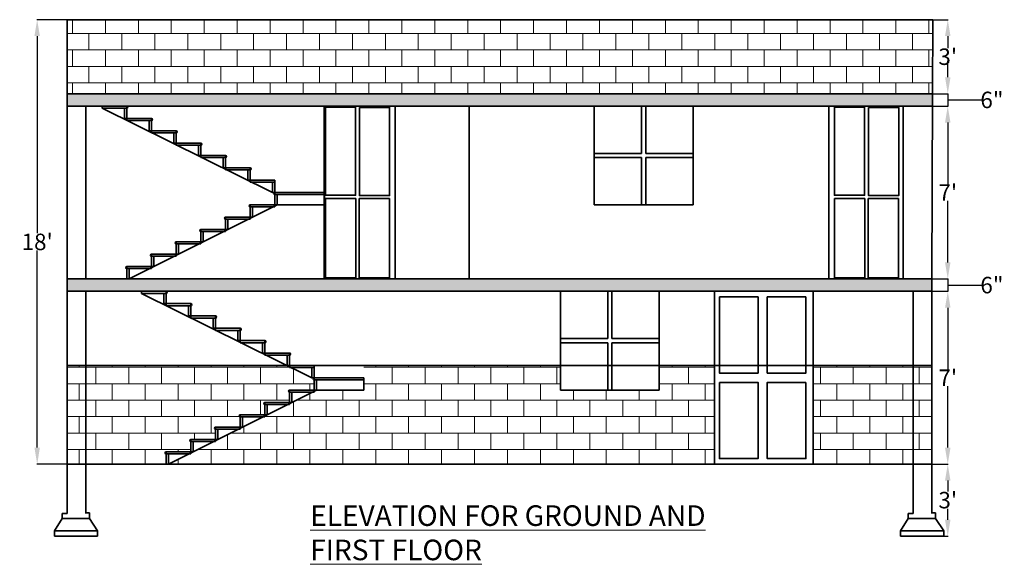
# Model space of a CAD drawing. Units: inches. Extents: x 179 to 2009, y 628 to 2084.
# Tile 5 of 5: x 1531 to 2009, y 888 to 1153. Entities that reach past the tile are written whole.
import ezdxf

# ---------------------------------------------------------------- set-up
doc = ezdxf.new("R2010")
doc.units = ezdxf.units.IN
doc.header["$MEASUREMENT"] = 0
for name, color, linetype, lineweight in [('A-ANNO-DIMS', 2, 'Continuous', 18), ('A-ANNO-TEXT', 7, 'Continuous', 18), ('A-ELEV', 7, 'Continuous', 35), ('A-ELEV-PATT', 8, 'Continuous', 13)]:
    doc.layers.add(name, color=color, linetype=linetype, lineweight=lineweight)
doc.styles.get("Standard").update_dxf_attribs({"font": 'arial.ttf'})
doc.dimstyles.get("Standard").update_dxf_attribs({"dimtxt": 8, "dimasz": 8, "dimexe": 0.18, "dimexo": 0.0625, "dimgap": 0.09, "dimtad": 0, "dimtih": 1, "dimtoh": 1, "dimdec": 0, "dimzin": 0, "dimdsep": 46, "dimlunit": 3, "dimtxsty": 'Standard', "dimcen": 0.09, "dimadec": 0, "dimazin": 0, "dimtfac": 1, "dimtdec": 0, "dimtofl": 0, "dimtmove": 0, "dimatfit": 3, "dimfxl": 1, "dimtolj": 1, "dimtzin": 0, "dimarcsym": 0})
pattern_1 = [(50, (0, 0), (7.172602, -0.627521), [0.75, -8.25]), (355, (0, 0), (-1.387513, 7.521921), [0.6, -6.6]), (100.45144, (0.598, -0.052), (5.785088, 6.8944), [0.637402, -7.01142]), (46.1842, (0, 2), (10.672413, -1.655193), [1.125, -12.375]), (96.63564, (0.889, 1.862), (9.34662, 9.741186), [0.956103, -10.51714]), (351.18416, (0, 2), (9.34662, 9.741186), [0.9, -9.9]), (21, (1, 1.5), (5.96907, -4.026189), [0.75, -8.25]), (326, (1, 1.5), (2.433153, 7.2515), [0.6, -6.6]), (71.45144, (1.4974, 1.1645), (8.402224, 3.225312), [0.637402, -7.01142]), (37.5, (0, 0), (0.1215986, 3.3289385), [0, -6.52, 0, -6.7, 0, -6.625]), (7.5, (0, 0), (2.6306954, 3.944117), [0, -3.82, 0, -6.37, 0, -2.525]), (327.5, (-2.23, 0), (5.3382244, -0.2255487), [0, -2.5, 0, -7.8, 0, -10.35]), (317.5, (-3.23, 0), (5.831862, 1.00105), [0, -3.25, 0, -5.18, 0, -7.35])]

# ---------------------------------------------------------------- blocks, each defined once
blk = doc.blocks.new('*D24')
at = {"layer": 'A-ANNO-DIMS', "color": 0, "lineweight": -2, "transparency": 16777216}
for p, q in [((1554.1, 1152.94), (1539.38, 1152.94)), ((1539.56, 1144.94), (1539.56, 1049.11)), ((1539.56, 944.94), (1539.56, 1040.76)), ((1554.1, 936.94), (1539.38, 936.94))]:
    blk.add_line(p, q, dxfattribs=at)
at = {"layer": 'A-ANNO-DIMS', "color": 0, "transparency": 16777216}
for points in [[(1538.22, 1144.94), (1540.89, 1144.94), (1539.56, 1152.94)], [(1538.22, 944.94), (1540.89, 944.94), (1539.56, 936.94)]]:
    blk.add_solid(points, dxfattribs=at)
at = {"layer": 'Defpoints', "color": 0, "transparency": 16777216}
for p in [(1554.16, 1152.94), (1539.56, 936.94), (1554.16, 936.94)]:
    blk.add_point(p, dxfattribs=at)
at = {"layer": 'A-ANNO-DIMS', "color": 0, "transparency": 16777216, "insert": (1539.56, 1044.94), "char_height": 8, "attachment_point": 5}
blk.add_mtext("\\A1;18'", dxfattribs=at)
blk = doc.blocks.new('*D25')
at = {"layer": 'A-ANNO-DIMS', "color": 0, "lineweight": -2, "transparency": 16777216}
for p, q in [((1974.69, 1152.94), (1982.07, 1152.94)), ((1981.89, 1144.94), (1981.89, 1139.11)), ((1981.89, 1124.94), (1981.89, 1130.76)), ((1974.69, 1116.94), (1982.07, 1116.94))]:
    blk.add_line(p, q, dxfattribs=at)
at = {"layer": 'A-ANNO-DIMS', "color": 0, "transparency": 16777216}
for points in [[(1980.56, 1144.94), (1983.22, 1144.94), (1981.89, 1152.94)], [(1980.56, 1124.94), (1983.22, 1124.94), (1981.89, 1116.94)]]:
    blk.add_solid(points, dxfattribs=at)
at = {"layer": 'Defpoints', "color": 0, "transparency": 16777216}
for p in [(1974.62, 1152.94), (1974.62, 1116.94), (1981.89, 1116.94)]:
    blk.add_point(p, dxfattribs=at)
at = {"layer": 'A-ANNO-DIMS', "color": 0, "transparency": 16777216, "insert": (1981.89, 1134.94), "char_height": 8, "attachment_point": 5}
blk.add_mtext("\\A1;3'", dxfattribs=at)
blk = doc.blocks.new('*D26')
at = {"layer": 'A-ANNO-DIMS', "color": 0, "lineweight": -2, "transparency": 16777216}
for p, q in [((1981.89, 1124.94), (1981.89, 1132.94)), ((1974.69, 1116.94), (1982.07, 1116.94)), ((1981.89, 1116.94), (1981.89, 1110.94)), ((1974.53, 1110.94), (1982.07, 1110.94)), ((1981.89, 1113.94), (1998.45, 1113.94)), ((1998.45, 1113.94), (1998.63, 1113.94)), ((1981.89, 1102.94), (1981.89, 1094.94))]:
    blk.add_line(p, q, dxfattribs=at)
at = {"layer": 'A-ANNO-DIMS', "color": 0, "transparency": 16777216}
for points in [[(1980.56, 1124.94), (1983.22, 1124.94), (1981.89, 1116.94)], [(1980.56, 1102.94), (1983.22, 1102.94), (1981.89, 1110.94)]]:
    blk.add_solid(points, dxfattribs=at)
at = {"layer": 'Defpoints', "color": 0, "transparency": 16777216}
for p in [(1974.62, 1116.94), (1974.47, 1110.94), (1981.89, 1110.94)]:
    blk.add_point(p, dxfattribs=at)
at = {"layer": 'A-ANNO-DIMS', "color": 0, "transparency": 16777216, "insert": (2003.34, 1113.94), "char_height": 8, "attachment_point": 5}
blk.add_mtext('\\A1;6"', dxfattribs=at)
blk = doc.blocks.new('*D27')
at = {"layer": 'A-ANNO-DIMS', "color": 0, "lineweight": -2, "transparency": 16777216}
for p, q in [((1974.53, 1110.94), (1982.07, 1110.94)), ((1981.89, 1102.94), (1981.89, 1073.03)), ((1981.89, 1034.94), (1981.89, 1064.85)), ((1974.22, 1026.94), (1982.07, 1026.94))]:
    blk.add_line(p, q, dxfattribs=at)
at = {"layer": 'A-ANNO-DIMS', "color": 0, "transparency": 16777216}
for points in [[(1980.56, 1102.94), (1983.22, 1102.94), (1981.89, 1110.94)], [(1980.56, 1034.94), (1983.22, 1034.94), (1981.89, 1026.94)]]:
    blk.add_solid(points, dxfattribs=at)
at = {"layer": 'Defpoints', "color": 0, "transparency": 16777216}
for p in [(1974.47, 1110.94), (1974.16, 1026.94), (1981.89, 1026.94)]:
    blk.add_point(p, dxfattribs=at)
at = {"layer": 'A-ANNO-DIMS', "color": 0, "transparency": 16777216, "insert": (1981.89, 1068.94), "char_height": 8, "attachment_point": 5}
blk.add_mtext("\\A1;7'", dxfattribs=at)
blk = doc.blocks.new('*D28')
at = {"layer": 'A-ANNO-DIMS', "color": 0, "lineweight": -2, "transparency": 16777216}
for p, q in [((1981.89, 1034.94), (1981.89, 1042.94)), ((1974.22, 1026.94), (1982.07, 1026.94)), ((1981.89, 1026.94), (1981.89, 1020.94)), ((1981.89, 1023.94), (1998.45, 1023.94)), ((1998.45, 1023.94), (1998.63, 1023.94)), ((1974.22, 1020.94), (1982.07, 1020.94)), ((1981.89, 1012.94), (1981.89, 1004.94))]:
    blk.add_line(p, q, dxfattribs=at)
at = {"layer": 'A-ANNO-DIMS', "color": 0, "transparency": 16777216}
for points in [[(1980.56, 1034.94), (1983.22, 1034.94), (1981.89, 1026.94)], [(1980.56, 1012.94), (1983.22, 1012.94), (1981.89, 1020.94)]]:
    blk.add_solid(points, dxfattribs=at)
at = {"layer": 'Defpoints', "color": 0, "transparency": 16777216}
for p in [(1974.16, 1026.94), (1974.16, 1020.94), (1981.89, 1020.94)]:
    blk.add_point(p, dxfattribs=at)
at = {"layer": 'A-ANNO-DIMS', "color": 0, "transparency": 16777216, "insert": (2003.34, 1023.94), "char_height": 8, "attachment_point": 5}
blk.add_mtext('\\A1;6"', dxfattribs=at)
blk = doc.blocks.new('*D29')
at = {"layer": 'A-ANNO-DIMS', "color": 0, "lineweight": -2, "transparency": 16777216}
for p, q in [((1974.22, 1020.94), (1982.07, 1020.94)), ((1981.89, 1012.94), (1981.89, 983.03)), ((1981.89, 944.94), (1981.89, 974.85)), ((1974.22, 936.94), (1982.07, 936.94))]:
    blk.add_line(p, q, dxfattribs=at)
at = {"layer": 'A-ANNO-DIMS', "color": 0, "transparency": 16777216}
for points in [[(1980.56, 1012.94), (1983.22, 1012.94), (1981.89, 1020.94)], [(1980.56, 944.94), (1983.22, 944.94), (1981.89, 936.94)]]:
    blk.add_solid(points, dxfattribs=at)
at = {"layer": 'Defpoints', "color": 0, "transparency": 16777216}
for p in [(1974.16, 1020.94), (1974.16, 936.94), (1981.89, 936.94)]:
    blk.add_point(p, dxfattribs=at)
at = {"layer": 'A-ANNO-DIMS', "color": 0, "transparency": 16777216, "insert": (1981.89, 978.94), "char_height": 8, "attachment_point": 5}
blk.add_mtext("\\A1;7'", dxfattribs=at)
blk = doc.blocks.new('*D30')
at = {"layer": 'A-ANNO-DIMS', "color": 0, "lineweight": -2, "transparency": 16777216}
for p, q in [((1974.22, 936.94), (1982.07, 936.94)), ((1981.89, 928.94), (1981.89, 923.61)), ((1981.89, 909.94), (1981.89, 915.26)), ((1977.81, 901.94), (1982.07, 901.94))]:
    blk.add_line(p, q, dxfattribs=at)
at = {"layer": 'A-ANNO-DIMS', "color": 0, "transparency": 16777216}
for points in [[(1980.56, 928.94), (1983.22, 928.94), (1981.89, 936.94)], [(1980.56, 909.94), (1983.22, 909.94), (1981.89, 901.94)]]:
    blk.add_solid(points, dxfattribs=at)
at = {"layer": 'Defpoints', "color": 0, "transparency": 16777216}
for p in [(1974.16, 936.94), (1977.75, 901.94), (1981.89, 901.94)]:
    blk.add_point(p, dxfattribs=at)
at = {"layer": 'A-ANNO-DIMS', "color": 0, "transparency": 16777216, "insert": (1981.89, 919.44), "char_height": 8, "attachment_point": 5}
blk.add_mtext("\\A1;3'", dxfattribs=at)

msp = doc.modelspace()

# ---------------------------------------------------------------- hatches: boundary and pattern name
at = {"layer": 'A-ELEV-PATT'}
h = msp.add_hatch(dxfattribs=at)
h.set_pattern_fill('AR-B816', color=256)
h.set_pattern_definition([(0, (500.695, 474.206), (0, 8), []), (90, (500.695, 474.206), (-8, 8), [8, -8])])
h.paths.add_polyline_path([(1974.49, 1116.94), (1974.62, 1152.94), (1554.16, 1152.94), (1554.16, 1116.94)])
h = msp.add_hatch(dxfattribs=at)
h.set_pattern_fill('AR-CONC', color=256)
h.set_pattern_definition(pattern_1)
h.paths.add_polyline_path([(1974.49, 1116.94), (1554.16, 1116.94), (1554.16, 1110.94), (1974.47, 1110.94)])
h = msp.add_hatch(dxfattribs=at)
h.set_pattern_fill('AR-CONC', color=256)
h.set_pattern_definition(pattern_1)
h.paths.add_polyline_path([(1974.16, 1026.94), (1554.16, 1026.94), (1554.16, 1020.94), (1974.16, 1020.94)])
h = msp.add_hatch(dxfattribs=at)
h.set_pattern_fill('AR-B816', color=256)
h.paths.add_polyline_path([(1650.16, 965.94, -1), (1650.16, 966.94), (1662.16, 966.94), (1662.16, 971.94, -1), (1662.16, 972.94), (1674.16, 972.94), (1674.16, 977.94, -1), (1674.16, 978.94), (1673.02, 978.94), (1662.92, 983.94), (1662.16, 983.94), (1662.16, 984.31), (1660.9, 984.94), (1563.16, 984.94), (1563.16, 936.94), (1602.16, 936.94), (1602.16, 941.94, -1), (1602.16, 942.94), (1614.16, 942.94), (1614.16, 947.94, -1), (1614.16, 948.94), (1626.16, 948.94), (1626.16, 953.94, -1), (1626.16, 954.94), (1638.16, 954.94), (1638.16, 959.94, -1), (1638.16, 960.94), (1650.16, 960.94)])
h.paths.add_polyline_path([(1698.16, 972.94), (1675.3, 972.94), (1674.16, 972.37), (1674.16, 971.94), (1673.3, 971.94), (1662.16, 966.37), (1662.16, 965.94), (1661.3, 965.94), (1650.16, 960.37), (1650.16, 959.94), (1649.3, 959.94), (1638.16, 954.37), (1638.16, 953.94), (1637.3, 953.94), (1626.16, 948.37), (1626.16, 947.94), (1625.3, 947.94), (1614.16, 942.37), (1614.16, 941.94), (1613.3, 941.94), (1603.3, 936.94), (1698.16, 936.94)])
h.paths.add_polyline_path([(1563.16, 984.94), (1554.16, 984.94), (1554.16, 936.94), (1563.16, 936.94)])
h.paths.add_polyline_path([(1868.5, 984.94), (1841.75, 984.94), (1841.75, 972.94), (1793.75, 972.94), (1793.75, 984.94), (1698.16, 984.94), (1698.16, 936.94), (1868.5, 936.94)])
h.paths.add_polyline_path([(1965.16, 984.94), (1916.5, 984.94), (1916.5, 936.94), (1965.16, 936.94)])
h.paths.add_polyline_path([(1974.16, 984.94), (1965.16, 984.94), (1965.16, 936.94), (1974.16, 936.94)])

# ---------------------------------------------------------------- linework, layer by layer
at = {"layer": 'A-ELEV'}
for p, q in [((1554.16, 1116.94), (1554.16, 1152.94)), ((1554.16, 1152.94), (1974.62, 1152.94)), ((1974.62, 1152.94), (1974.49, 1116.94)), ((1554.16, 1116.94), (1974.49, 1116.94)), ((1554.16, 1116.94), (1554.16, 1026.94)), ((1974.49, 1116.94), (1974.16, 1026.94)), ((1554.16, 1110.94), (1974.47, 1110.94)), ((1563.16, 1026.94), (1563.16, 1110.94)), ((1583.07, 1110.94), (1571.07, 1110.94)), ((1571.07, 1110.94), (1571.07, 1109.94)), ((1571.07, 1109.94), (1583.07, 1109.94)), ((1571.07, 1109.94), (1653.94, 1068.94)), ((1581.94, 1109.94), (1581.94, 1104.94)), ((1583.07, 1104.94), (1583.07, 1110.94)), ((1678.94, 1026.94), (1678.94, 1110.94)), ((1713.45, 1026.94), (1713.45, 1110.94)), ((1749.45, 1026.94), (1749.45, 1110.94)), ((1810.16, 1062.94), (1810.16, 1110.94)), ((1833.16, 1087.94), (1833.16, 1110.94)), ((1835.16, 1087.94), (1835.16, 1110.94)), ((1858.16, 1062.94), (1858.16, 1110.94)), ((1924.18, 1026.94), (1924.18, 1110.94)), ((1960.18, 1026.94), (1960.18, 1110.94)), ((1583.07, 1104.94), (1581.94, 1104.94)), ((1595.07, 1104.94), (1583.07, 1104.94)), ((1583.07, 1104.94), (1583.07, 1103.94)), ((1595.07, 1098.94), (1595.07, 1104.94)), ((1583.07, 1103.94), (1595.07, 1103.94)), ((1593.94, 1103.94), (1593.94, 1098.94)), ((1595.07, 1098.94), (1593.94, 1098.94)), ((1607.07, 1098.94), (1595.07, 1098.94)), ((1595.07, 1098.94), (1595.07, 1097.94)), ((1595.07, 1097.94), (1607.07, 1097.94)), ((1605.94, 1097.94), (1605.94, 1092.94)), ((1607.07, 1092.94), (1607.07, 1098.94)), ((1607.07, 1092.94), (1605.94, 1092.94)), ((1619.07, 1092.94), (1607.07, 1092.94)), ((1607.07, 1092.94), (1607.07, 1091.94)), ((1607.07, 1091.94), (1619.07, 1091.94)), ((1617.94, 1091.94), (1617.94, 1086.94)), ((1619.07, 1086.94), (1619.07, 1092.94)), ((1619.07, 1086.94), (1617.94, 1086.94)), ((1631.07, 1086.94), (1619.07, 1086.94)), ((1619.07, 1086.94), (1619.07, 1085.94)), ((1619.07, 1085.94), (1631.07, 1085.94)), ((1629.94, 1085.94), (1629.94, 1080.94)), ((1631.07, 1080.94), (1631.07, 1086.94)), ((1833.16, 1087.94), (1810.16, 1087.94)), ((1833.16, 1085.94), (1810.16, 1085.94)), ((1833.16, 1062.94), (1833.16, 1085.94)), ((1858.16, 1087.94), (1835.16, 1087.94)), ((1835.16, 1062.94), (1835.16, 1085.94)), ((1858.16, 1085.94), (1835.16, 1085.94)), ((1631.07, 1080.94), (1629.94, 1080.94)), ((1643.07, 1080.94), (1631.07, 1080.94)), ((1631.07, 1080.94), (1631.07, 1079.94)), ((1631.07, 1079.94), (1643.07, 1079.94)), ((1641.94, 1079.94), (1641.94, 1074.94)), ((1643.07, 1074.94), (1643.07, 1080.94)), ((1643.07, 1074.94), (1641.94, 1074.94)), ((1655.07, 1074.94), (1643.07, 1074.94)), ((1643.07, 1074.94), (1643.07, 1073.94)), ((1643.07, 1073.94), (1655.07, 1073.94)), ((1653.94, 1073.94), (1653.94, 1068.94)), ((1655.07, 1068.94), (1655.07, 1074.94)), ((1655.07, 1068.94), (1653.94, 1068.94)), ((1655.07, 1062.94), (1655.07, 1068.94)), ((1655.07, 1068.94), (1667.07, 1068.94)), ((1667.07, 1067.94), (1655.07, 1067.94)), ((1656.21, 1067.94), (1656.21, 1062.94)), ((1667.07, 1068.94), (1679.07, 1068.94)), ((1667.07, 1067.94), (1679.07, 1067.94)), ((1679.07, 1068.94), (1679.07, 1062.94)), ((1584.21, 1026.94), (1656.21, 1062.94)), ((1643.07, 1056.94), (1643.07, 1062.94)), ((1643.07, 1062.94), (1655.07, 1062.94)), ((1655.07, 1061.94), (1643.07, 1061.94)), ((1644.21, 1061.94), (1644.21, 1056.94)), ((1655.07, 1062.94), (1655.07, 1061.94)), ((1655.07, 1062.94), (1656.21, 1062.94)), ((1656.21, 1062.94), (1679.07, 1062.94)), ((1810.16, 1062.94), (1858.16, 1062.94)), ((1631.07, 1050.94), (1631.07, 1056.94)), ((1631.07, 1056.94), (1643.07, 1056.94)), ((1643.07, 1055.94), (1631.07, 1055.94)), ((1632.21, 1055.94), (1632.21, 1050.94)), ((1643.07, 1056.94), (1643.07, 1055.94)), ((1643.07, 1056.94), (1644.21, 1056.94)), ((1619.07, 1044.94), (1619.07, 1050.94)), ((1619.07, 1050.94), (1631.07, 1050.94)), ((1631.07, 1049.94), (1619.07, 1049.94)), ((1620.21, 1049.94), (1620.21, 1044.94)), ((1631.07, 1050.94), (1631.07, 1049.94)), ((1631.07, 1050.94), (1632.21, 1050.94)), ((1607.07, 1038.94), (1607.07, 1044.94)), ((1607.07, 1044.94), (1619.07, 1044.94)), ((1619.07, 1043.94), (1607.07, 1043.94)), ((1608.21, 1043.94), (1608.21, 1038.94)), ((1619.07, 1044.94), (1619.07, 1043.94)), ((1619.07, 1044.94), (1620.21, 1044.94)), ((1595.07, 1032.94), (1595.07, 1038.94)), ((1595.07, 1038.94), (1607.07, 1038.94)), ((1607.07, 1037.94), (1595.07, 1037.94)), ((1596.21, 1037.94), (1596.21, 1032.94)), ((1607.07, 1038.94), (1607.07, 1037.94)), ((1607.07, 1038.94), (1608.21, 1038.94)), ((1583.07, 1026.94), (1583.07, 1032.94)), ((1583.07, 1032.94), (1595.07, 1032.94)), ((1595.07, 1031.94), (1583.07, 1031.94)), ((1584.21, 1031.94), (1584.21, 1026.94)), ((1595.07, 1032.94), (1595.07, 1031.94)), ((1595.07, 1032.94), (1596.21, 1032.94)), ((1554.16, 1026.94), (1974.16, 1026.94)), ((1554.16, 1026.94), (1554.16, 936.94)), ((1554.16, 1026.94), (1974.16, 1026.94)), ((1583.07, 1026.94), (1584.21, 1026.94)), ((1974.16, 1026.94), (1974.16, 936.94)), ((1554.16, 1020.94), (1974.16, 1020.94)), ((1563.16, 936.94), (1563.16, 1020.94)), ((1602.16, 1020.94), (1590.16, 1020.94)), ((1590.16, 1020.94), (1590.16, 1019.94)), ((1590.16, 1019.94), (1602.16, 1019.94)), ((1590.16, 1019.94), (1673.02, 978.94)), ((1601.02, 1019.94), (1601.02, 1014.94)), ((1602.16, 1014.94), (1602.16, 1020.94)), ((1793.75, 972.94), (1793.75, 1020.94)), ((1816.75, 997.94), (1816.75, 1020.94)), ((1818.75, 997.94), (1818.75, 1020.94)), ((1841.75, 972.94), (1841.75, 1020.94)), ((1868.5, 936.94), (1868.5, 1020.94)), ((1916.5, 936.94), (1916.5, 1020.94)), ((1965.16, 936.94), (1965.16, 1020.94)), ((1602.16, 1014.94), (1601.02, 1014.94)), ((1614.16, 1014.94), (1602.16, 1014.94)), ((1602.16, 1014.94), (1602.16, 1013.94)), ((1614.16, 1008.94), (1614.16, 1014.94)), ((1602.16, 1013.94), (1614.16, 1013.94)), ((1613.02, 1013.94), (1613.02, 1008.94)), ((1614.16, 1008.94), (1613.02, 1008.94)), ((1626.16, 1008.94), (1614.16, 1008.94)), ((1614.16, 1008.94), (1614.16, 1007.94)), ((1614.16, 1007.94), (1626.16, 1007.94)), ((1625.02, 1007.94), (1625.02, 1002.94)), ((1626.16, 1002.94), (1626.16, 1008.94)), ((1626.16, 1002.94), (1625.02, 1002.94)), ((1638.16, 1002.94), (1626.16, 1002.94)), ((1626.16, 1002.94), (1626.16, 1001.94)), ((1626.16, 1001.94), (1638.16, 1001.94)), ((1637.02, 1001.94), (1637.02, 996.94)), ((1638.16, 996.94), (1638.16, 1002.94)), ((1638.16, 996.94), (1637.02, 996.94)), ((1650.16, 996.94), (1638.16, 996.94)), ((1638.16, 996.94), (1638.16, 995.94)), ((1638.16, 995.94), (1650.16, 995.94)), ((1649.02, 995.94), (1649.02, 990.94)), ((1650.16, 990.94), (1650.16, 996.94)), ((1816.75, 997.94), (1793.75, 997.94)), ((1816.75, 995.94), (1793.75, 995.94)), ((1816.75, 972.94), (1816.75, 995.94)), ((1841.75, 997.94), (1818.75, 997.94)), ((1818.75, 972.94), (1818.75, 995.94)), ((1841.75, 995.94), (1818.75, 995.94)), ((1650.16, 990.94), (1649.02, 990.94)), ((1662.16, 990.94), (1650.16, 990.94)), ((1650.16, 990.94), (1650.16, 989.94)), ((1662.16, 984.94), (1662.16, 990.94)), ((1650.16, 989.94), (1662.16, 989.94)), ((1661.02, 989.94), (1661.02, 984.94)), ((1554.16, 984.94), (1974.16, 984.94)), ((1662.16, 984.94), (1661.02, 984.94)), ((1674.16, 984.94), (1662.16, 984.94)), ((1662.16, 984.94), (1662.16, 983.94)), ((1662.16, 983.94), (1674.16, 983.94)), ((1673.02, 983.94), (1673.02, 978.94)), ((1674.16, 978.94), (1674.16, 984.94)), ((1674.16, 978.94), (1673.02, 978.94)), ((1674.16, 972.94), (1674.16, 978.94)), ((1674.16, 978.94), (1686.16, 978.94)), ((1686.16, 977.94), (1674.16, 977.94)), ((1675.3, 977.94), (1675.3, 972.94)), ((1686.16, 978.94), (1698.16, 978.94)), ((1686.16, 977.94), (1698.16, 977.94)), ((1698.16, 978.94), (1698.16, 972.94)), ((1603.3, 936.94), (1675.3, 972.94)), ((1662.16, 966.94), (1662.16, 972.94)), ((1662.16, 972.94), (1674.16, 972.94)), ((1674.16, 971.94), (1662.16, 971.94)), ((1663.3, 971.94), (1663.3, 966.94)), ((1674.16, 972.94), (1674.16, 971.94)), ((1674.16, 972.94), (1675.3, 972.94)), ((1675.3, 972.94), (1698.16, 972.94)), ((1793.75, 972.94), (1841.75, 972.94)), ((1650.16, 960.94), (1650.16, 966.94)), ((1650.16, 966.94), (1662.16, 966.94)), ((1662.16, 966.94), (1662.16, 965.94)), ((1662.16, 966.94), (1663.3, 966.94)), ((1662.16, 965.94), (1650.16, 965.94)), ((1651.3, 965.94), (1651.3, 960.94)), ((1638.16, 954.94), (1638.16, 960.94)), ((1638.16, 960.94), (1650.16, 960.94)), ((1650.16, 959.94), (1638.16, 959.94)), ((1639.3, 959.94), (1639.3, 954.94)), ((1650.16, 960.94), (1650.16, 959.94)), ((1650.16, 960.94), (1651.3, 960.94)), ((1626.16, 948.94), (1626.16, 954.94)), ((1626.16, 954.94), (1638.16, 954.94)), ((1638.16, 953.94), (1626.16, 953.94)), ((1627.3, 953.94), (1627.3, 948.94)), ((1638.16, 954.94), (1638.16, 953.94)), ((1638.16, 954.94), (1639.3, 954.94)), ((1614.16, 942.94), (1614.16, 948.94)), ((1614.16, 948.94), (1626.16, 948.94)), ((1626.16, 947.94), (1614.16, 947.94)), ((1615.3, 947.94), (1615.3, 942.94)), ((1626.16, 948.94), (1626.16, 947.94)), ((1626.16, 948.94), (1627.3, 948.94)), ((1602.16, 936.94), (1602.16, 942.94)), ((1602.16, 942.94), (1614.16, 942.94)), ((1614.16, 942.94), (1614.16, 941.94)), ((1614.16, 942.94), (1615.3, 942.94)), ((1614.16, 941.94), (1602.16, 941.94)), ((1603.3, 941.94), (1603.3, 936.94)), ((1554.16, 936.94), (1974.16, 936.94)), ((1554.16, 936.94), (1554.16, 912.94)), ((1563.16, 936.94), (1563.16, 912.94)), ((1602.16, 936.94), (1603.3, 936.94)), ((1965.16, 936.94), (1965.16, 912.94)), ((1974.16, 936.94), (1974.16, 912.94)), ((1551.68, 910.51), (1547.95, 904.45)), ((1554.16, 912.94), (1551.68, 912.94)), ((1551.68, 912.94), (1551.68, 910.51)), ((1551.68, 910.51), (1564.99, 910.51)), ((1564.99, 913.22), (1563.16, 913.22)), ((1564.99, 910.51), (1564.99, 913.22)), ((1568.94, 904.45), (1564.99, 910.51)), ((1962.68, 910.51), (1958.95, 904.45)), ((1965.16, 912.94), (1962.68, 912.94)), ((1962.68, 912.94), (1962.68, 910.51)), ((1962.68, 910.51), (1975.99, 910.51)), ((1975.99, 913.22), (1974.16, 913.22)), ((1975.99, 910.51), (1975.99, 913.22)), ((1979.94, 904.45), (1975.99, 910.51)), ((1547.95, 904.45), (1568.94, 904.45)), ((1547.95, 904.45), (1547.95, 901.94)), ((1568.93, 901.94), (1568.93, 904.45)), ((1958.95, 904.45), (1979.94, 904.45)), ((1958.95, 904.45), (1958.95, 901.94)), ((1979.93, 901.94), (1979.93, 904.45)), ((1547.95, 901.94), (1568.93, 901.94)), ((1958.95, 901.94), (1979.93, 901.94))]:
    msp.add_line(p, q, dxfattribs=at)
for points in [[(1679.55, 1110.42), (1694.2, 1110.42), (1694.2, 1067.58), (1679.55, 1067.58)], [(1696.13, 1110.32), (1710.78, 1110.32), (1710.78, 1067.48), (1696.13, 1067.48)], [(1926.84, 1110.42), (1941.49, 1110.42), (1941.49, 1067.58), (1926.84, 1067.58)], [(1943.42, 1110.32), (1958.06, 1110.32), (1958.06, 1067.48), (1943.42, 1067.48)], [(1679.59, 1066.02), (1694.28, 1066.02), (1694.28, 1027.5), (1679.59, 1027.5)], [(1695.94, 1066.02), (1710.63, 1066.02), (1710.63, 1027.5), (1695.94, 1027.5)], [(1926.88, 1066.02), (1941.57, 1066.02), (1941.57, 1027.5), (1926.88, 1027.5)], [(1943.23, 1066.02), (1957.92, 1066.02), (1957.92, 1027.5), (1943.23, 1027.5)], [(1870.96, 1018.21), (1889.73, 1018.21), (1889.73, 981.17), (1870.96, 981.17)], [(1912.95, 1018.21), (1894.18, 1018.21), (1894.18, 981.17), (1912.95, 981.17)], [(1870.96, 976.65), (1889.73, 976.65), (1889.73, 939.61), (1870.96, 939.61)], [(1912.95, 976.65), (1894.18, 976.65), (1894.18, 939.61), (1912.95, 939.61)]]:
    msp.add_lwpolyline(points, close=True, dxfattribs=at)
for centre, start, end in [((1583.07, 1110.44), 270, 90), ((1595.07, 1104.44), 270, 90), ((1607.07, 1098.44), 270, 90), ((1619.07, 1092.44), 270, 90), ((1631.07, 1086.44), 270, 90), ((1643.07, 1080.44), 270, 90), ((1655.07, 1068.44), 90, 270), ((1643.07, 1062.44), 90, 270), ((1631.07, 1056.44), 90, 270), ((1619.07, 1050.44), 90, 270), ((1607.07, 1044.44), 90, 270), ((1595.07, 1038.44), 90, 270), ((1583.07, 1032.44), 90, 270), ((1602.16, 1020.44), 270, 90), ((1614.16, 1014.44), 270, 90), ((1626.16, 1008.44), 270, 90), ((1638.16, 1002.44), 270, 90), ((1650.16, 996.44), 270, 90), ((1662.16, 990.44), 270, 90), ((1674.16, 978.44), 90, 270), ((1662.16, 972.44), 90, 270), ((1650.16, 966.44), 90, 270), ((1638.16, 960.44), 90, 270), ((1626.16, 954.44), 90, 270), ((1614.16, 948.44), 90, 270), ((1602.16, 942.44), 90, 270)]:
    msp.add_arc(centre, 0.5, start, end, dxfattribs=at)

# ---------------------------------------------------------------- texts
at = {"layer": 'A-ANNO-TEXT', "insert": (1672.18, 916.91), "char_height": 10, "attachment_point": 1}
msp.add_mtext_dynamic_manual_height_columns('{\\fArial|b1|i0|c0|p34;\\LELEVATION FOR GROUND AND FIRST FLOOR}', width=224.9889, gutter_width=1, heights=[0], dxfattribs=at)

# ---------------------------------------------------------------- dimensions: what is measured, and where the dimension line sits
at = {"layer": 'A-ANNO-DIMS'}
for base, p1, p2, override, picture, middle in [((1539.56, 936.94), (1554.16, 1152.94), (1554.16, 936.94), {"dimclrd": 0, "dimclre": 0, "dimclrt": 0}, '*D24', (1539.56, 1044.94)), ((1981.89, 1116.94), (1974.62, 1152.94), (1974.62, 1116.94), {"dimclrd": 0, "dimclre": 0, "dimclrt": 0}, '*D25', (1981.89, 1134.94)), ((1981.89, 1110.94), (1974.62, 1116.94), (1974.47, 1110.94), {"dimclrd": 0, "dimclre": 0, "dimclrt": 0, "dimtmove": 1}, '*D26', (1998.72, 1113.94)), ((1981.89, 1026.94), (1974.47, 1110.94), (1974.16, 1026.94), {"dimclrd": 0, "dimclre": 0, "dimclrt": 0, "dimtmove": 1}, '*D27', (1981.89, 1068.94)), ((1981.89, 1020.94), (1974.16, 1026.94), (1974.16, 1020.94), {"dimclrd": 0, "dimclre": 0, "dimclrt": 0, "dimtmove": 1}, '*D28', (1998.72, 1023.94)), ((1981.89, 936.94), (1974.16, 1020.94), (1974.16, 936.94), {"dimclrd": 0, "dimclre": 0, "dimclrt": 0, "dimtmove": 1}, '*D29', (1981.89, 978.94))]:
    dim = msp.add_linear_dim(base=base, p1=p1, p2=p2, angle=90, dimstyle='Standard', override=override, dxfattribs=at)
    dim.commit()
    dim.dimension.update_dxf_attribs({"geometry": picture, "text_midpoint": middle})
dim = msp.add_linear_dim(base=(1981.89, 901.94), p1=(1974.16, 936.94), p2=(1977.75, 901.94), angle=90, text="3'", dimstyle='Standard', override={"dimclrd": 0, "dimclre": 0, "dimclrt": 0, "dimtmove": 1}, dxfattribs=at)
dim.commit()
dim.dimension.update_dxf_attribs({"geometry": '*D30', "text_midpoint": (1981.89, 919.44)})

doc.saveas('drawing.dxf')
